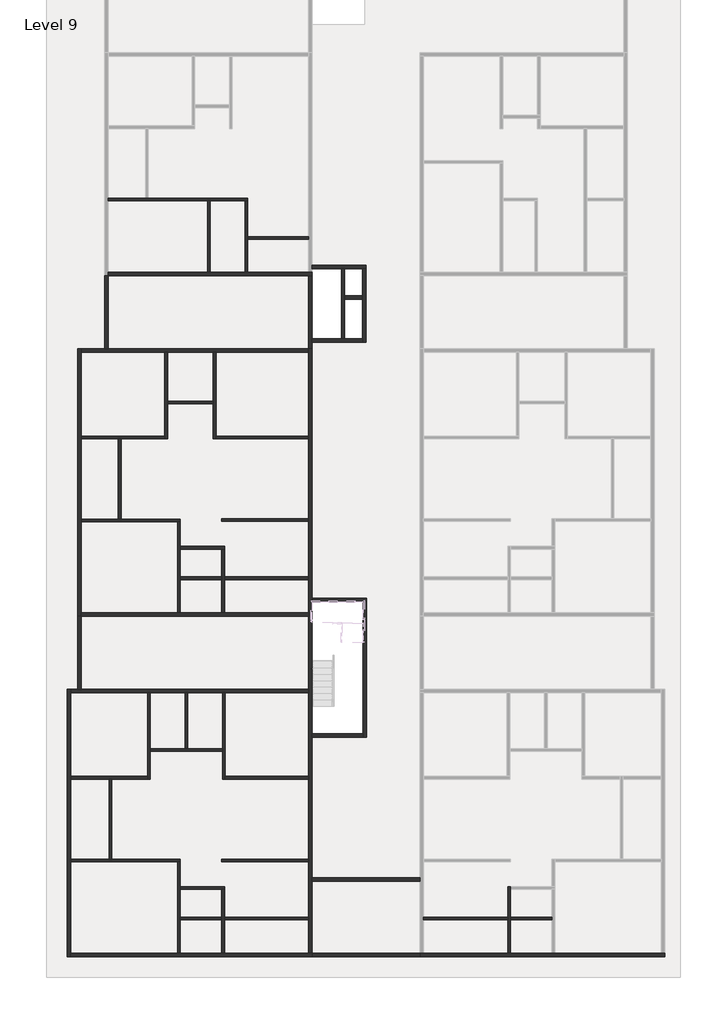
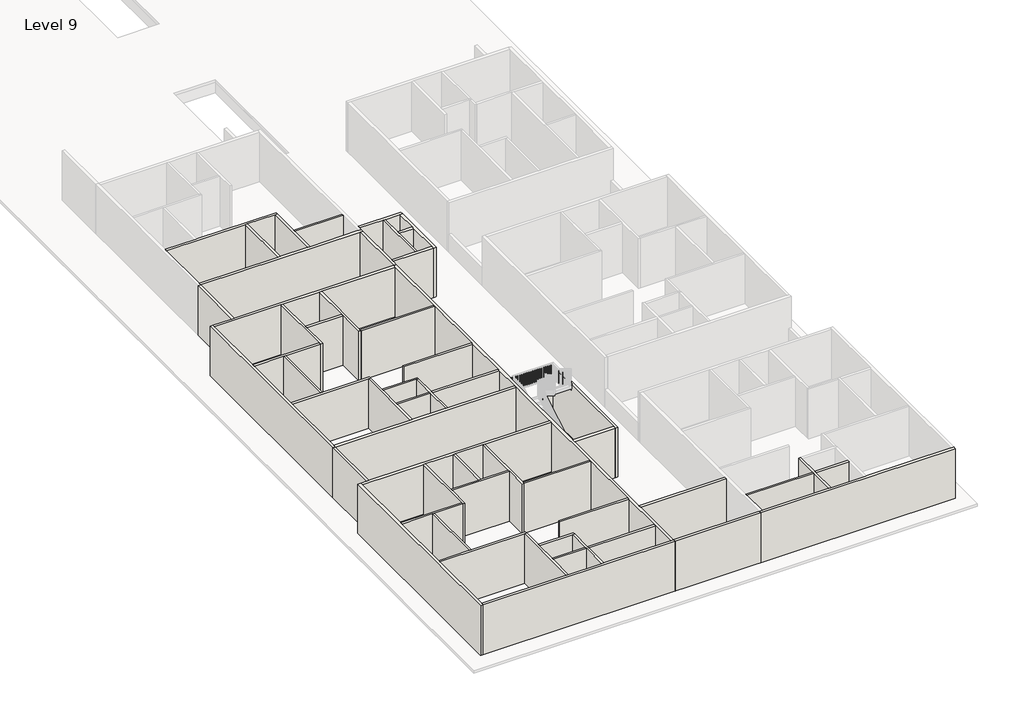
# One storey, part 1 of 8: 55 walls.
"""IFC4 building model written with IfcOpenShell, lengths in millimetres."""

from ifc_helpers import new_model, si_unit, frame, origin, place, context, project, spatial, polyline, outline, extrude, faceted_brep, element, save

model = new_model("IFC4")

# Units and contexts
model_context = context("Model", 3, world=origin())
ifc_project = project(units=[si_unit("LENGTHUNIT", "METRE", prefix="MILLI")], contexts=[model_context])

# Site, building, storey
site = spatial("IfcSite", under=ifc_project)
building = spatial("IfcBuilding", under=site)
storey = spatial("IfcBuildingStorey", under=building, Name="Level 9", Elevation=49618.6172466)

# Walls
placement = place(None, origin())
element("IfcWall", 1, ObjectType="4.5\"", at=placement, inside=storey, context=model_context, shape_type="Brep", body=[
    faceted_brep([(-12531.5544854, -1061.7344126, 49618.6172466), (-8188.1544854, -1061.7344126, 49618.6172466), (-8073.8544854, -1061.7344126, 49618.6172466), (-6549.8544854, -1061.7344126, 49618.6172466), (-6435.5544854, -1061.7344126, 49618.6172466), (-6435.5544854, -1061.7344126, 52666.6172466), (-6549.8544854, -1061.7344126, 52666.6172466), (-8073.8544854, -1061.7344126, 52666.6172466), (-8188.1544854, -1061.7344126, 52666.6172466), (-12531.5544854, -1061.7344126, 52666.6172466), (-12531.5544854, -947.4344126, 49618.6172466), (-12531.5544854, -947.4344126, 52666.6172466), (-10907.2415084, -947.4344126, 52666.6172466), (-10792.9415084, -947.4344126, 52666.6172466), (-6435.5544854, -947.4344126, 52666.6172466), (-6435.5544854, -947.4344126, 49618.6172466), (-10792.9415084, -947.4344126, 49618.6172466), (-10907.2415084, -947.4344126, 49618.6172466)], [[[0, 1, 2, 3, 4, 5, 6, 7, 8, 9]], [[10, 11, 12, 13, 14, 15, 16, 17]], [[4, 3, 2, 1, 0, 10, 17, 16, 15]], [[0, 9, 11, 10]], [[5, 4, 15, 14]], [[9, 8, 7, 6, 5, 14, 13, 12, 11]]]),
])
element("IfcWall", 2, ObjectType="4.5\"", at=placement, inside=storey, context=model_context, shape_type="Brep", body=[
    faceted_brep([(-6549.8544854, -1061.7344126, 49618.6172466), (-6549.8544854, -4185.9344126, 49618.6172466), (-6549.8544854, -4185.9344126, 52666.6172466), (-6549.8544854, -1061.7344126, 52666.6172466), (-6435.5544854, -1061.7344126, 49618.6172466), (-6435.5544854, -1061.7344126, 52666.6172466), (-6435.5544854, -2623.8344126, 52666.6172466), (-6435.5544854, -2738.1344126, 52666.6172466), (-6435.5544854, -4185.9344126, 52666.6172466), (-6435.5544854, -4185.9344126, 49618.6172466), (-6435.5544854, -2738.1344126, 49618.6172466), (-6435.5544854, -2623.8344126, 49618.6172466)], [[[0, 1, 2, 3]], [[4, 5, 6, 7, 8, 9, 10, 11]], [[1, 0, 4, 11, 10, 9]], [[0, 3, 5, 4]], [[2, 1, 9, 8]], [[3, 2, 8, 7, 6, 5]]]),
])
element("IfcWall", 3, ObjectType="4.5\"", at=placement, inside=storey, context=model_context, shape_type="SweptSolid", body=[
    extrude(outline(polyline([(-8188.1544854, -4185.9344126), (-8188.1544854, -1061.7344126), (-8073.8544854, -1061.7344126), (-8073.8544854, -4185.9344126), (-8188.1544854, -4185.9344126)])), frame((0.0, 0.0, 49618.6172466), z_axis=(0.0, 0.0, 1.0), x_axis=(1.0, 0.0, 0.0)), (0.0, 0.0, 1.0), 3048.0),
])
element("IfcWall", 4, ObjectType="4.5\"", at=placement, inside=storey, context=model_context, shape_type="SweptSolid", body=[
    extrude(outline(polyline([(-6435.5544854, -2623.8344126), (-3769.8415084, -2623.8344126), (-3769.8415084, -2738.1344126), (-6435.5544854, -2738.1344126), (-6435.5544854, -2623.8344126)])), frame((0.0, 0.0, 49618.6172466), z_axis=(0.0, 0.0, 1.0), x_axis=(1.0, 0.0, 0.0)), (0.0, 0.0, 1.0), 3048.0),
])
element("IfcWall", 5, ObjectType="4.5\"", at=placement, inside=storey, context=model_context, shape_type="Brep", body=[
    faceted_brep([(-10061.4044854, -7691.1344126, 49618.6172466), (-10061.4044854, -11348.7344126, 49618.6172466), (-10061.4044854, -11463.0344126, 49618.6172466), (-10061.4044854, -11463.0344126, 52666.6172466), (-10061.4044854, -11348.7344126, 52666.6172466), (-10061.4044854, -7691.1344126, 52666.6172466), (-9947.1044854, -7691.1344126, 49618.6172466), (-9947.1044854, -7691.1344126, 52666.6172466), (-9947.1044854, -9824.7344126, 52666.6172466), (-9947.1044854, -9939.0344126, 52666.6172466), (-9947.1044854, -11463.0344126, 52666.6172466), (-9947.1044854, -11463.0344126, 49618.6172466), (-9947.1044854, -9939.0344126, 49618.6172466), (-9947.1044854, -9824.7344126, 49618.6172466)], [[[0, 1, 2, 3, 4, 5]], [[6, 7, 8, 9, 10, 11, 12, 13]], [[2, 1, 0, 6, 13, 12, 11]], [[0, 5, 7, 6]], [[3, 2, 11, 10]], [[5, 4, 3, 10, 9, 8, 7]]]),
])
element("IfcWall", 6, ObjectType="4.5\"", at=placement, inside=storey, context=model_context, shape_type="Brep", body=[
    faceted_brep([(-10061.4044854, -11348.7344126, 49618.6172466), (-13719.0044854, -11348.7344126, 49618.6172466), (-13719.0044854, -11348.7344126, 52666.6172466), (-10061.4044854, -11348.7344126, 52666.6172466), (-10061.4044854, -11463.0344126, 49618.6172466), (-10061.4044854, -11463.0344126, 52666.6172466), (-11980.3915084, -11463.0344126, 52666.6172466), (-12094.6915084, -11463.0344126, 52666.6172466), (-13719.0044854, -11463.0344126, 52666.6172466), (-13719.0044854, -11463.0344126, 49618.6172466), (-12094.6915084, -11463.0344126, 49618.6172466), (-11980.3915084, -11463.0344126, 49618.6172466)], [[[0, 1, 2, 3]], [[4, 5, 6, 7, 8, 9, 10, 11]], [[1, 0, 4, 11, 10, 9]], [[0, 3, 5, 4]], [[2, 1, 9, 8]], [[3, 2, 8, 7, 6, 5]]]),
])
element("IfcWall", 7, ObjectType="4.5\"", at=placement, inside=storey, context=model_context, shape_type="SweptSolid", body=[
    extrude(outline(polyline([(-12094.6915084, -14968.2344126), (-12094.6915084, -11463.0344126), (-11980.3915084, -11463.0344126), (-11980.3915084, -14968.2344126), (-12094.6915084, -14968.2344126)])), frame((0.0, 0.0, 49618.6172466), z_axis=(0.0, 0.0, 1.0), x_axis=(1.0, 0.0, 0.0)), (0.0, 0.0, 1.0), 3048.0),
])
element("IfcWall", 8, ObjectType="4.5\"", at=placement, inside=storey, context=model_context, shape_type="Brep", body=[
    faceted_brep([(-13719.0044854, -15095.2344126, 49618.6172466), (-9510.2415084, -15095.2344126, 49618.6172466), (-9395.9415084, -15095.2344126, 49618.6172466), (-9395.9415084, -15095.2344126, 52666.6172466), (-9510.2415084, -15095.2344126, 52666.6172466), (-13719.0044854, -15095.2344126, 52666.6172466), (-13719.0044854, -14980.9344126, 49618.6172466), (-13719.0044854, -14980.9344126, 52666.6172466), (-9395.9415084, -14980.9344126, 52666.6172466), (-9395.9415084, -14980.9344126, 49618.6172466)], [[[0, 1, 2, 3, 4, 5]], [[6, 7, 8, 9]], [[2, 1, 0, 6, 9]], [[0, 5, 7, 6]], [[3, 2, 9, 8]], [[5, 4, 3, 8, 7]]]),
])
element("IfcWall", 9, ObjectType="4.5\"", at=placement, inside=storey, context=model_context, shape_type="Brep", body=[
    faceted_brep([(-9510.2415084, -15095.2344126, 49618.6172466), (-9510.2415084, -19070.3344126, 49618.6172466), (-9510.2415084, -19070.3344126, 52666.6172466), (-9510.2415084, -15095.2344126, 52666.6172466), (-9395.9415084, -15095.2344126, 49618.6172466), (-9395.9415084, -15095.2344126, 52666.6172466), (-9395.9415084, -16174.7344126, 52666.6172466), (-9395.9415084, -16289.0344126, 52666.6172466), (-9395.9415084, -17508.2344126, 52666.6172466), (-9395.9415084, -17622.5344126, 52666.6172466), (-9395.9415084, -19070.3344126, 52666.6172466), (-9395.9415084, -19070.3344126, 49618.6172466), (-9395.9415084, -17622.5344126, 49618.6172466), (-9395.9415084, -17508.2344126, 49618.6172466), (-9395.9415084, -16289.0344126, 49618.6172466), (-9395.9415084, -16174.7344126, 49618.6172466)], [[[0, 1, 2, 3]], [[4, 5, 6, 7, 8, 9, 10, 11, 12, 13, 14, 15]], [[1, 0, 4, 15, 14, 13, 12, 11]], [[0, 3, 5, 4]], [[2, 1, 11, 10]], [[3, 2, 10, 9, 8, 7, 6, 5]]]),
])
element("IfcWall", 10, ObjectType="4.5\"", at=placement, inside=storey, context=model_context, shape_type="Brep", body=[
    faceted_brep([(-9395.9415084, -16289.0344126, 49618.6172466), (-7567.1415084, -16289.0344126, 49618.6172466), (-7452.8415084, -16289.0344126, 49618.6172466), (-7452.8415084, -16289.0344126, 52666.6172466), (-7567.1415084, -16289.0344126, 52666.6172466), (-9395.9415084, -16289.0344126, 52666.6172466), (-9395.9415084, -16174.7344126, 49618.6172466), (-9395.9415084, -16174.7344126, 52666.6172466), (-7452.8415084, -16174.7344126, 52666.6172466), (-7452.8415084, -16174.7344126, 49618.6172466)], [[[0, 1, 2, 3, 4, 5]], [[6, 7, 8, 9]], [[2, 1, 0, 6, 9]], [[0, 5, 7, 6]], [[3, 2, 9, 8]], [[5, 4, 3, 8, 7]]]),
])
element("IfcWall", 11, ObjectType="4.5\"", at=placement, inside=storey, context=model_context, shape_type="Brep", body=[
    faceted_brep([(-7567.1415084, -16289.0344126, 49618.6172466), (-7567.1415084, -17508.2344126, 49618.6172466), (-7567.1415084, -17622.5344126, 49618.6172466), (-7567.1415084, -19070.3344126, 49618.6172466), (-7567.1415084, -19070.3344126, 52666.6172466), (-7567.1415084, -17622.5344126, 52666.6172466), (-7567.1415084, -17508.2344126, 52666.6172466), (-7567.1415084, -16289.0344126, 52666.6172466), (-7452.8415084, -16289.0344126, 49618.6172466), (-7452.8415084, -16289.0344126, 52666.6172466), (-7452.8415084, -17508.2344126, 52666.6172466), (-7452.8415084, -17622.5344126, 52666.6172466), (-7452.8415084, -19070.3344126, 52666.6172466), (-7452.8415084, -19070.3344126, 49618.6172466), (-7452.8415084, -17622.5344126, 49618.6172466), (-7452.8415084, -17508.2344126, 49618.6172466)], [[[0, 1, 2, 3, 4, 5, 6, 7]], [[8, 9, 10, 11, 12, 13, 14, 15]], [[3, 2, 1, 0, 8, 15, 14, 13]], [[0, 7, 9, 8]], [[4, 3, 13, 12]], [[7, 6, 5, 4, 12, 11, 10, 9]]]),
])
element("IfcWall", 12, ObjectType="4.5\"", at=placement, inside=storey, context=model_context, shape_type="SweptSolid", body=[
    extrude(outline(polyline([(-7567.1415084, -17622.5344126), (-9395.9415084, -17622.5344126), (-9395.9415084, -17508.2344126), (-7567.1415084, -17508.2344126), (-7567.1415084, -17622.5344126)])), frame((0.0, 0.0, 49618.6172466), z_axis=(0.0, 0.0, 1.0), x_axis=(1.0, 0.0, 0.0)), (0.0, 0.0, 1.0), 3048.0),
])
element("IfcWall", 13, ObjectType="4.5\"", at=placement, inside=storey, context=model_context, shape_type="SweptSolid", body=[
    extrude(outline(polyline([(-3769.8415084, -17622.5344126), (-7452.8415084, -17622.5344126), (-7452.8415084, -17508.2344126), (-3769.8415084, -17508.2344126), (-3769.8415084, -17622.5344126)])), frame((0.0, 0.0, 49618.6172466), z_axis=(0.0, 0.0, 1.0), x_axis=(1.0, 0.0, 0.0)), (0.0, 0.0, 1.0), 3048.0),
])
element("IfcWall", 14, ObjectType="4.5\"", at=placement, inside=storey, context=model_context, shape_type="SweptSolid", body=[
    extrude(outline(polyline([(-7567.1415084, -14968.2344126), (-3769.8415084, -14968.2344126), (-3769.8415084, -15082.5344126), (-7567.1415084, -15082.5344126), (-7567.1415084, -14968.2344126)])), frame((0.0, 0.0, 49618.6172466), z_axis=(0.0, 0.0, 1.0), x_axis=(1.0, 0.0, 0.0)), (0.0, 0.0, 1.0), 3048.0),
])
element("IfcWall", 15, ObjectType="4.5\"", at=placement, inside=storey, context=model_context, shape_type="SweptSolid", body=[
    extrude(outline(polyline([(-7940.5044854, -9939.0344126), (-9947.1044854, -9939.0344126), (-9947.1044854, -9824.7344126), (-7940.5044854, -9824.7344126), (-7940.5044854, -9939.0344126)])), frame((0.0, 0.0, 49618.6172466), z_axis=(0.0, 0.0, 1.0), x_axis=(1.0, 0.0, 0.0)), (0.0, 0.0, 1.0), 3048.0),
])
element("IfcWall", 16, ObjectType="4.5\"", at=placement, inside=storey, context=model_context, shape_type="Brep", body=[
    faceted_brep([(-7940.5044854, -7691.1344126, 49618.6172466), (-7940.5044854, -9824.7344126, 49618.6172466), (-7940.5044854, -9939.0344126, 49618.6172466), (-7940.5044854, -11463.0344126, 49618.6172466), (-7940.5044854, -11463.0344126, 52666.6172466), (-7940.5044854, -9939.0344126, 52666.6172466), (-7940.5044854, -9824.7344126, 52666.6172466), (-7940.5044854, -7691.1344126, 52666.6172466), (-7826.2044854, -7691.1344126, 49618.6172466), (-7826.2044854, -7691.1344126, 52666.6172466), (-7826.2044854, -11348.7344126, 52666.6172466), (-7826.2044854, -11463.0344126, 52666.6172466), (-7826.2044854, -11463.0344126, 49618.6172466), (-7826.2044854, -11348.7344126, 49618.6172466)], [[[0, 1, 2, 3, 4, 5, 6, 7]], [[8, 9, 10, 11, 12, 13]], [[3, 2, 1, 0, 8, 13, 12]], [[0, 7, 9, 8]], [[4, 3, 12, 11]], [[7, 6, 5, 4, 11, 10, 9]]]),
])
element("IfcWall", 17, ObjectType="4.5\"", at=placement, inside=storey, context=model_context, shape_type="SweptSolid", body=[
    extrude(outline(polyline([(-3769.8415084, -11463.0344126), (-7826.2044854, -11463.0344126), (-7826.2044854, -11348.7344126), (-3769.8415084, -11348.7344126), (-3769.8415084, -11463.0344126)])), frame((0.0, 0.0, 49618.6172466), z_axis=(0.0, 0.0, 1.0), x_axis=(1.0, 0.0, 0.0)), (0.0, 0.0, 1.0), 3048.0),
])
element("IfcWall", 18, ObjectType="4.5\"", at=placement, inside=storey, context=model_context, shape_type="Brep", body=[
    faceted_brep([(-10818.3415084, -22575.5344126, 49618.6172466), (-10818.3415084, -26233.1344126, 49618.6172466), (-10818.3415084, -26347.4344126, 49618.6172466), (-10818.3415084, -26347.4344126, 52666.6172466), (-10818.3415084, -26233.1344126, 52666.6172466), (-10818.3415084, -22575.5344126, 52666.6172466), (-10704.0415084, -22575.5344126, 49618.6172466), (-10704.0415084, -22575.5344126, 52666.6172466), (-10704.0415084, -25013.9344126, 52666.6172466), (-10704.0415084, -25128.2344126, 52666.6172466), (-10704.0415084, -26347.4344126, 52666.6172466), (-10704.0415084, -26347.4344126, 49618.6172466), (-10704.0415084, -25128.2344126, 49618.6172466), (-10704.0415084, -25013.9344126, 49618.6172466)], [[[0, 1, 2, 3, 4, 5]], [[6, 7, 8, 9, 10, 11, 12, 13]], [[2, 1, 0, 6, 13, 12, 11]], [[0, 5, 7, 6]], [[3, 2, 11, 10]], [[5, 4, 3, 10, 9, 8, 7]]]),
])
element("IfcWall", 19, ObjectType="4.5\"", at=placement, inside=storey, context=model_context, shape_type="Brep", body=[
    faceted_brep([(-10818.3415084, -26233.1344126, 49618.6172466), (-14171.1415084, -26233.1344126, 49618.6172466), (-14171.1415084, -26233.1344126, 52666.6172466), (-10818.3415084, -26233.1344126, 52666.6172466), (-10818.3415084, -26347.4344126, 49618.6172466), (-10818.3415084, -26347.4344126, 52666.6172466), (-12380.4415084, -26347.4344126, 52666.6172466), (-12494.7415084, -26347.4344126, 52666.6172466), (-14171.1415084, -26347.4344126, 52666.6172466), (-14171.1415084, -26347.4344126, 49618.6172466), (-12494.7415084, -26347.4344126, 49618.6172466), (-12380.4415084, -26347.4344126, 49618.6172466)], [[[0, 1, 2, 3]], [[4, 5, 6, 7, 8, 9, 10, 11]], [[1, 0, 4, 11, 10, 9]], [[0, 3, 5, 4]], [[2, 1, 9, 8]], [[3, 2, 8, 7, 6, 5]]]),
])
element("IfcWall", 20, ObjectType="4.5\"", at=placement, inside=storey, context=model_context, shape_type="SweptSolid", body=[
    extrude(outline(polyline([(-9180.0415084, -25013.9344126), (-9180.0415084, -22575.5344126), (-9065.7415084, -22575.5344126), (-9065.7415084, -25013.9344126), (-9180.0415084, -25013.9344126)])), frame((0.0, 0.0, 49618.6172466), z_axis=(0.0, 0.0, 1.0), x_axis=(1.0, 0.0, 0.0)), (0.0, 0.0, 1.0), 3048.0),
])
element("IfcWall", 21, ObjectType="4.5\"", at=placement, inside=storey, context=model_context, shape_type="Brep", body=[
    faceted_brep([(-10704.0415084, -25128.2344126, 49618.6172466), (-7541.7415084, -25128.2344126, 49618.6172466), (-7541.7415084, -25128.2344126, 52666.6172466), (-10704.0415084, -25128.2344126, 52666.6172466), (-10704.0415084, -25013.9344126, 49618.6172466), (-10704.0415084, -25013.9344126, 52666.6172466), (-9180.0415084, -25013.9344126, 52666.6172466), (-9065.7415084, -25013.9344126, 52666.6172466), (-7541.7415084, -25013.9344126, 52666.6172466), (-7541.7415084, -25013.9344126, 49618.6172466), (-9065.7415084, -25013.9344126, 49618.6172466), (-9180.0415084, -25013.9344126, 49618.6172466)], [[[0, 1, 2, 3]], [[4, 5, 6, 7, 8, 9, 10, 11]], [[1, 0, 4, 11, 10, 9]], [[0, 3, 5, 4]], [[2, 1, 9, 8]], [[3, 2, 8, 7, 6, 5]]]),
])
element("IfcWall", 22, ObjectType="4.5\"", at=placement, inside=storey, context=model_context, shape_type="Brep", body=[
    faceted_brep([(-7541.7415084, -22575.5344126, 49618.6172466), (-7541.7415084, -25013.9344126, 49618.6172466), (-7541.7415084, -25128.2344126, 49618.6172466), (-7541.7415084, -26347.4344126, 49618.6172466), (-7541.7415084, -26347.4344126, 52666.6172466), (-7541.7415084, -25128.2344126, 52666.6172466), (-7541.7415084, -25013.9344126, 52666.6172466), (-7541.7415084, -22575.5344126, 52666.6172466), (-7427.4415084, -22575.5344126, 49618.6172466), (-7427.4415084, -22575.5344126, 52666.6172466), (-7427.4415084, -26233.1344126, 52666.6172466), (-7427.4415084, -26347.4344126, 52666.6172466), (-7427.4415084, -26347.4344126, 49618.6172466), (-7427.4415084, -26233.1344126, 49618.6172466)], [[[0, 1, 2, 3, 4, 5, 6, 7]], [[8, 9, 10, 11, 12, 13]], [[3, 2, 1, 0, 8, 13, 12]], [[0, 7, 9, 8]], [[4, 3, 12, 11]], [[7, 6, 5, 4, 11, 10, 9]]]),
])
element("IfcWall", 23, ObjectType="4.5\"", at=placement, inside=storey, context=model_context, shape_type="SweptSolid", body=[
    extrude(outline(polyline([(-3769.8415084, -26347.4344126), (-7427.4415084, -26347.4344126), (-7427.4415084, -26233.1344126), (-3769.8415084, -26233.1344126), (-3769.8415084, -26347.4344126)])), frame((0.0, 0.0, 49618.6172466), z_axis=(0.0, 0.0, 1.0), x_axis=(1.0, 0.0, 0.0)), (0.0, 0.0, 1.0), 3048.0),
])
element("IfcWall", 24, ObjectType="4.5\"", at=placement, inside=storey, context=model_context, shape_type="SweptSolid", body=[
    extrude(outline(polyline([(-12494.7415084, -29852.6344126), (-12494.7415084, -26347.4344126), (-12380.4415084, -26347.4344126), (-12380.4415084, -29852.6344126), (-12494.7415084, -29852.6344126)])), frame((0.0, 0.0, 49618.6172466), z_axis=(0.0, 0.0, 1.0), x_axis=(1.0, 0.0, 0.0)), (0.0, 0.0, 1.0), 3048.0),
])
element("IfcWall", 25, ObjectType="4.5\"", at=placement, inside=storey, context=model_context, shape_type="Brep", body=[
    faceted_brep([(-14171.1415084, -29966.9344126, 49618.6172466), (-9510.2415084, -29966.9344126, 49618.6172466), (-9395.9415084, -29966.9344126, 49618.6172466), (-9395.9415084, -29966.9344126, 52666.6172466), (-9510.2415084, -29966.9344126, 52666.6172466), (-14171.1415084, -29966.9344126, 52666.6172466), (-14171.1415084, -29852.6344126, 49618.6172466), (-14171.1415084, -29852.6344126, 52666.6172466), (-12494.7415084, -29852.6344126, 52666.6172466), (-12380.4415084, -29852.6344126, 52666.6172466), (-9395.9415084, -29852.6344126, 52666.6172466), (-9395.9415084, -29852.6344126, 49618.6172466), (-12380.4415084, -29852.6344126, 49618.6172466), (-12494.7415084, -29852.6344126, 49618.6172466)], [[[0, 1, 2, 3, 4, 5]], [[6, 7, 8, 9, 10, 11, 12, 13]], [[2, 1, 0, 6, 13, 12, 11]], [[0, 5, 7, 6]], [[3, 2, 11, 10]], [[5, 4, 3, 10, 9, 8, 7]]]),
])
element("IfcWall", 26, ObjectType="4.5\"", at=placement, inside=storey, context=model_context, shape_type="Brep", body=[
    faceted_brep([(-9510.2415084, -29966.9344126, 49618.6172466), (-9510.2415084, -33954.7344126, 49618.6172466), (-9510.2415084, -33954.7344126, 52666.6172466), (-9510.2415084, -29966.9344126, 52666.6172466), (-9395.9415084, -29966.9344126, 49618.6172466), (-9395.9415084, -29966.9344126, 52666.6172466), (-9395.9415084, -31059.1344126, 52666.6172466), (-9395.9415084, -31173.4344126, 52666.6172466), (-9395.9415084, -32392.6344126, 52666.6172466), (-9395.9415084, -32506.9344126, 52666.6172466), (-9395.9415084, -33954.7344126, 52666.6172466), (-9395.9415084, -33954.7344126, 49618.6172466), (-9395.9415084, -32506.9344126, 49618.6172466), (-9395.9415084, -32392.6344126, 49618.6172466), (-9395.9415084, -31173.4344126, 49618.6172466), (-9395.9415084, -31059.1344126, 49618.6172466)], [[[0, 1, 2, 3]], [[4, 5, 6, 7, 8, 9, 10, 11, 12, 13, 14, 15]], [[1, 0, 4, 15, 14, 13, 12, 11]], [[0, 3, 5, 4]], [[2, 1, 11, 10]], [[3, 2, 10, 9, 8, 7, 6, 5]]]),
])
element("IfcWall", 27, ObjectType="4.5\"", at=placement, inside=storey, context=model_context, shape_type="Brep", body=[
    faceted_brep([(-9395.9415084, -31173.4344126, 49618.6172466), (-7567.1415084, -31173.4344126, 49618.6172466), (-7452.8415084, -31173.4344126, 49618.6172466), (-7452.8415084, -31173.4344126, 52666.6172466), (-7567.1415084, -31173.4344126, 52666.6172466), (-9395.9415084, -31173.4344126, 52666.6172466), (-9395.9415084, -31059.1344126, 49618.6172466), (-9395.9415084, -31059.1344126, 52666.6172466), (-7452.8415084, -31059.1344126, 52666.6172466), (-7452.8415084, -31059.1344126, 49618.6172466)], [[[0, 1, 2, 3, 4, 5]], [[6, 7, 8, 9]], [[2, 1, 0, 6, 9]], [[0, 5, 7, 6]], [[3, 2, 9, 8]], [[5, 4, 3, 8, 7]]]),
])
element("IfcWall", 28, ObjectType="4.5\"", at=placement, inside=storey, context=model_context, shape_type="Brep", body=[
    faceted_brep([(-7567.1415084, -31173.4344126, 49618.6172466), (-7567.1415084, -32392.6344126, 49618.6172466), (-7567.1415084, -32506.9344126, 49618.6172466), (-7567.1415084, -33954.7344126, 49618.6172466), (-7567.1415084, -33954.7344126, 52666.6172466), (-7567.1415084, -32506.9344126, 52666.6172466), (-7567.1415084, -32392.6344126, 52666.6172466), (-7567.1415084, -31173.4344126, 52666.6172466), (-7452.8415084, -31173.4344126, 49618.6172466), (-7452.8415084, -31173.4344126, 52666.6172466), (-7452.8415084, -32392.6344126, 52666.6172466), (-7452.8415084, -32506.9344126, 52666.6172466), (-7452.8415084, -33954.7344126, 52666.6172466), (-7452.8415084, -33954.7344126, 49618.6172466), (-7452.8415084, -32506.9344126, 49618.6172466), (-7452.8415084, -32392.6344126, 49618.6172466)], [[[0, 1, 2, 3, 4, 5, 6, 7]], [[8, 9, 10, 11, 12, 13, 14, 15]], [[3, 2, 1, 0, 8, 15, 14, 13]], [[0, 7, 9, 8]], [[4, 3, 13, 12]], [[7, 6, 5, 4, 12, 11, 10, 9]]]),
])
element("IfcWall", 29, ObjectType="4.5\"", at=placement, inside=storey, context=model_context, shape_type="SweptSolid", body=[
    extrude(outline(polyline([(-3769.8415084, -32392.6344126), (-3769.8415084, -32506.9344126), (-7452.8415084, -32506.9344126), (-7452.8415084, -32392.6344126), (-3769.8415084, -32392.6344126)])), frame((0.0, 0.0, 49618.6172466), z_axis=(0.0, 0.0, 1.0), x_axis=(1.0, 0.0, 0.0)), (0.0, 0.0, 1.0), 3048.0),
    extrude(outline(polyline([(-9395.9415084, -32506.9344126), (-9395.9415084, -32392.6344126), (-7567.1415084, -32392.6344126), (-7567.1415084, -32506.9344126), (-9395.9415084, -32506.9344126)])), frame((0.0, 0.0, 49618.6172466), z_axis=(0.0, 0.0, 1.0), x_axis=(1.0, 0.0, 0.0)), (0.0, 0.0, 1.0), 3048.0),
])
element("IfcWall", 30, ObjectType="4.5\"", at=placement, inside=storey, context=model_context, shape_type="SweptSolid", body=[
    extrude(outline(polyline([(-7567.1415084, -29852.6344126), (-3769.8415084, -29852.6344126), (-3769.8415084, -29966.9344126), (-7567.1415084, -29966.9344126), (-7567.1415084, -29852.6344126)])), frame((0.0, 0.0, 49618.6172466), z_axis=(0.0, 0.0, 1.0), x_axis=(1.0, 0.0, 0.0)), (0.0, 0.0, 1.0), 3048.0),
])
element("IfcWall", 31, ObjectType="4.5\"", at=placement, inside=storey, context=model_context, shape_type="SweptSolid", body=[
    extrude(outline(polyline([(4942.3584916, -32506.9344126), (1259.3584916, -32506.9344126), (1259.3584916, -32392.6344126), (4942.3584916, -32392.6344126), (4942.3584916, -32506.9344126)])), frame((0.0, 0.0, 49618.6172466), z_axis=(0.0, 0.0, 1.0), x_axis=(1.0, 0.0, 0.0)), (0.0, 0.0, 1.0), 3048.0),
])
element("IfcWall", 32, ObjectType="4.5\"", at=placement, inside=storey, context=model_context, shape_type="Brep", body=[
    faceted_brep([(4942.3584916, -31059.1344126, 49618.6172466), (4942.3584916, -32392.6344126, 49618.6172466), (4942.3584916, -32506.9344126, 49618.6172466), (4942.3584916, -33954.7344126, 49618.6172466), (4942.3584916, -33954.7344126, 52666.6172466), (4942.3584916, -32506.9344126, 52666.6172466), (4942.3584916, -32392.6344126, 52666.6172466), (4942.3584916, -31059.1344126, 52666.6172466), (5056.6584916, -31059.1344126, 49618.6172466), (5056.6584916, -31059.1344126, 52666.6172466), (5056.6584916, -31173.4344126, 52666.6172466), (5056.6584916, -32392.6344126, 52666.6172466), (5056.6584916, -32506.9344126, 52666.6172466), (5056.6584916, -33954.7344126, 52666.6172466), (5056.6584916, -33954.7344126, 49618.6172466), (5056.6584916, -32506.9344126, 49618.6172466), (5056.6584916, -32392.6344126, 49618.6172466), (5056.6584916, -31173.4344126, 49618.6172466)], [[[0, 1, 2, 3, 4, 5, 6, 7]], [[8, 9, 10, 11, 12, 13, 14, 15, 16, 17]], [[3, 2, 1, 0, 8, 17, 16, 15, 14]], [[4, 3, 14, 13]], [[0, 7, 9, 8]], [[7, 6, 5, 4, 13, 12, 11, 10, 9]]]),
])
element("IfcWall", 33, ObjectType="4.5\"", at=placement, inside=storey, context=model_context, shape_type="SweptSolid", body=[
    extrude(outline(polyline([(6885.4584916, -32506.9344126), (5056.6584916, -32506.9344126), (5056.6584916, -32392.6344126), (6885.4584916, -32392.6344126), (6885.4584916, -32506.9344126)])), frame((0.0, 0.0, 49618.6172466), z_axis=(0.0, 0.0, 1.0), x_axis=(1.0, 0.0, 0.0)), (0.0, 0.0, 1.0), 3048.0),
])
element("IfcWall", 34, ObjectType="4.5\"", at=placement, inside=storey, context=model_context, shape_type="Brep", body=[
    faceted_brep([(-2207.6738684, -7082.6751812, 49618.6172466), (-2207.6738684, -5366.3479894, 49618.6172466), (-2207.6738684, -5213.9479894, 49618.6172466), (-2207.6738684, -4034.6751812, 49618.6172466), (-2207.6738684, -4034.6751812, 52666.6172466), (-2207.6738684, -5213.9479894, 52666.6172466), (-2207.6738684, -5366.3479894, 52666.6172466), (-2207.6738684, -7082.6751812, 52666.6172466), (-2321.9738684, -7082.6751812, 49618.6172466), (-2321.9738684, -7082.6751812, 52666.6172466), (-2321.9738684, -4034.6751812, 52666.6172466), (-2321.9738684, -4034.6751812, 49618.6172466)], [[[0, 1, 2, 3, 4, 5, 6, 7]], [[8, 9, 10, 11]], [[3, 2, 1, 0, 8, 11]], [[7, 6, 5, 4, 10, 9]], [[4, 3, 11, 10]], [[0, 7, 9, 8]]]),
])
element("IfcWall", 35, ObjectType="6\"", at=placement, inside=storey, context=model_context, shape_type="Brep", body=[
    faceted_brep([(-12531.5544854, -4338.3344126, 49618.6172466), (-3769.8415084, -4338.3344126, 49618.6172466), (-3617.4415084, -4338.3344126, 49618.6172466), (-3617.4415084, -4338.3344126, 52666.6172466), (-3769.8415084, -4338.3344126, 52666.6172466), (-12531.5544854, -4338.3344126, 52666.6172466), (-12531.5544854, -4185.9344126, 49618.6172466), (-12531.5544854, -4185.9344126, 52666.6172466), (-8188.1544854, -4185.9344126, 52666.6172466), (-8073.8544854, -4185.9344126, 52666.6172466), (-6549.8544854, -4185.9344126, 52666.6172466), (-6435.5544854, -4185.9344126, 52666.6172466), (-3769.8415084, -4185.9344126, 52666.6172466), (-3617.4415084, -4185.9344126, 52666.6172466), (-3617.4415084, -4185.9344126, 49618.6172466), (-3769.8415084, -4185.9344126, 49618.6172466), (-6435.5544854, -4185.9344126, 49618.6172466), (-6549.8544854, -4185.9344126, 49618.6172466), (-8073.8544854, -4185.9344126, 49618.6172466), (-8188.1544854, -4185.9344126, 49618.6172466)], [[[0, 1, 2, 3, 4, 5]], [[6, 7, 8, 9, 10, 11, 12, 13, 14, 15, 16, 17, 18, 19]], [[2, 1, 0, 6, 19, 18, 17, 16, 15, 14]], [[0, 5, 7, 6]], [[3, 2, 14, 13]], [[5, 4, 3, 13, 12, 11, 10, 9, 8, 7]]]),
])
element("IfcWall", 36, ObjectType="6\"", at=placement, inside=storey, context=model_context, shape_type="Brep", body=[
    faceted_brep([(-13871.4044854, -7538.7344126, 49618.6172466), (-13871.4044854, -19222.7344126, 49618.6172466), (-13871.4044854, -19222.7344126, 52666.6172466), (-13871.4044854, -7538.7344126, 52666.6172466), (-13719.0044854, -7538.7344126, 49618.6172466), (-13719.0044854, -7538.7344126, 52666.6172466), (-13719.0044854, -7691.1344126, 52666.6172466), (-13719.0044854, -11348.7344126, 52666.6172466), (-13719.0044854, -11463.0344126, 52666.6172466), (-13719.0044854, -14980.9344126, 52666.6172466), (-13719.0044854, -15095.2344126, 52666.6172466), (-13719.0044854, -19070.3344126, 52666.6172466), (-13719.0044854, -19222.7344126, 52666.6172466), (-13719.0044854, -19222.7344126, 49618.6172466), (-13719.0044854, -19070.3344126, 49618.6172466), (-13719.0044854, -15095.2344126, 49618.6172466), (-13719.0044854, -14980.9344126, 49618.6172466), (-13719.0044854, -11463.0344126, 49618.6172466), (-13719.0044854, -11348.7344126, 49618.6172466), (-13719.0044854, -7691.1344126, 49618.6172466)], [[[0, 1, 2, 3]], [[4, 5, 6, 7, 8, 9, 10, 11, 12, 13, 14, 15, 16, 17, 18, 19]], [[1, 0, 4, 19, 18, 17, 16, 15, 14, 13]], [[2, 1, 13, 12]], [[0, 3, 5, 4]], [[3, 2, 12, 11, 10, 9, 8, 7, 6, 5]]]),
])
element("IfcWall", 37, ObjectType="6\"", at=placement, inside=storey, context=model_context, shape_type="Brep", body=[
    faceted_brep([(-13719.0044854, -19222.7344126, 49618.6172466), (-3769.8415084, -19222.7344126, 49618.6172466), (-3769.8415084, -19222.7344126, 52666.6172466), (-13719.0044854, -19222.7344126, 52666.6172466), (-13719.0044854, -19070.3344126, 49618.6172466), (-13719.0044854, -19070.3344126, 52666.6172466), (-9510.2415084, -19070.3344126, 52666.6172466), (-9395.9415084, -19070.3344126, 52666.6172466), (-7567.1415084, -19070.3344126, 52666.6172466), (-7452.8415084, -19070.3344126, 52666.6172466), (-3769.8415084, -19070.3344126, 52666.6172466), (-3769.8415084, -19070.3344126, 49618.6172466), (-7452.8415084, -19070.3344126, 49618.6172466), (-7567.1415084, -19070.3344126, 49618.6172466), (-9395.9415084, -19070.3344126, 49618.6172466), (-9510.2415084, -19070.3344126, 49618.6172466)], [[[0, 1, 2, 3]], [[4, 5, 6, 7, 8, 9, 10, 11, 12, 13, 14, 15]], [[1, 0, 4, 15, 14, 13, 12, 11]], [[0, 3, 5, 4]], [[2, 1, 11, 10]], [[3, 2, 10, 9, 8, 7, 6, 5]]]),
])
element("IfcWall", 38, ObjectType="6\"", at=placement, inside=storey, context=model_context, shape_type="Brep", body=[
    faceted_brep([(-3617.4415084, -33954.7344126, 49618.6172466), (-3617.4415084, -30820.9325185, 49618.6172466), (-3617.4415084, -30668.5325185, 49618.6172466), (-3617.4415084, -24525.9851539, 49618.6172466), (-3617.4415084, -24373.5851539, 49618.6172466), (-3617.4415084, -18582.3851539, 49618.6172466), (-3617.4415084, -18429.9851539, 49618.6172466), (-3617.4415084, -7538.7344126, 49618.6172466), (-3617.4415084, -7538.7344126, 52666.6172466), (-3617.4415084, -18429.9851539, 52666.6172466), (-3617.4415084, -18582.3851539, 52666.6172466), (-3617.4415084, -24373.5851539, 52666.6172466), (-3617.4415084, -24525.9851539, 52666.6172466), (-3617.4415084, -30668.5325185, 52666.6172466), (-3617.4415084, -30820.9325185, 52666.6172466), (-3617.4415084, -33954.7344126, 52666.6172466), (-3769.8415084, -33954.7344126, 49618.6172466), (-3769.8415084, -33954.7344126, 52666.6172466), (-3769.8415084, -32506.9344126, 52666.6172466), (-3769.8415084, -32392.6344126, 52666.6172466), (-3769.8415084, -29966.9344126, 52666.6172466), (-3769.8415084, -29852.6344126, 52666.6172466), (-3769.8415084, -26347.4344126, 52666.6172466), (-3769.8415084, -26233.1344126, 52666.6172466), (-3769.8415084, -22575.5344126, 52666.6172466), (-3769.8415084, -22423.1344126, 52666.6172466), (-3769.8415084, -19222.7344126, 52666.6172466), (-3769.8415084, -19070.3344126, 52666.6172466), (-3769.8415084, -17622.5344126, 52666.6172466), (-3769.8415084, -17508.2344126, 52666.6172466), (-3769.8415084, -15082.5344126, 52666.6172466), (-3769.8415084, -14968.2344126, 52666.6172466), (-3769.8415084, -11463.0344126, 52666.6172466), (-3769.8415084, -11348.7344126, 52666.6172466), (-3769.8415084, -7691.1344126, 52666.6172466), (-3769.8415084, -7538.7344126, 52666.6172466), (-3769.8415084, -7538.7344126, 49618.6172466), (-3769.8415084, -7691.1344126, 49618.6172466), (-3769.8415084, -11348.7344126, 49618.6172466), (-3769.8415084, -11463.0344126, 49618.6172466), (-3769.8415084, -14968.2344126, 49618.6172466), (-3769.8415084, -15082.5344126, 49618.6172466), (-3769.8415084, -17508.2344126, 49618.6172466), (-3769.8415084, -17622.5344126, 49618.6172466), (-3769.8415084, -19070.3344126, 49618.6172466), (-3769.8415084, -19222.7344126, 49618.6172466), (-3769.8415084, -22423.1344126, 49618.6172466), (-3769.8415084, -22575.5344126, 49618.6172466), (-3769.8415084, -26233.1344126, 49618.6172466), (-3769.8415084, -26347.4344126, 49618.6172466), (-3769.8415084, -29852.6344126, 49618.6172466), (-3769.8415084, -29966.9344126, 49618.6172466), (-3769.8415084, -32392.6344126, 49618.6172466), (-3769.8415084, -32506.9344126, 49618.6172466)], [[[0, 1, 2, 3, 4, 5, 6, 7, 8, 9, 10, 11, 12, 13, 14, 15]], [[16, 17, 18, 19, 20, 21, 22, 23, 24, 25, 26, 27, 28, 29, 30, 31, 32, 33, 34, 35, 36, 37, 38, 39, 40, 41, 42, 43, 44, 45, 46, 47, 48, 49, 50, 51, 52, 53]], [[7, 6, 5, 4, 3, 2, 1, 0, 16, 53, 52, 51, 50, 49, 48, 47, 46, 45, 44, 43, 42, 41, 40, 39, 38, 37, 36]], [[8, 7, 36, 35]], [[0, 15, 17, 16]], [[15, 14, 13, 12, 11, 10, 9, 8, 35, 34, 33, 32, 31, 30, 29, 28, 27, 26, 25, 24, 23, 22, 21, 20, 19, 18, 17]]]),
])
element("IfcWall", 39, ObjectType="6\"", at=placement, inside=storey, context=model_context, shape_type="Brep", body=[
    faceted_brep([(-3769.8415084, -7538.7344126, 49618.6172466), (-12531.5544854, -7538.7344126, 49618.6172466), (-12683.9544854, -7538.7344126, 49618.6172466), (-13719.0044854, -7538.7344126, 49618.6172466), (-13719.0044854, -7538.7344126, 52666.6172466), (-12683.9544854, -7538.7344126, 52666.6172466), (-12531.5544854, -7538.7344126, 52666.6172466), (-3769.8415084, -7538.7344126, 52666.6172466), (-3769.8415084, -7691.1344126, 49618.6172466), (-3769.8415084, -7691.1344126, 52666.6172466), (-7826.2044854, -7691.1344126, 52666.6172466), (-7940.5044854, -7691.1344126, 52666.6172466), (-9947.1044854, -7691.1344126, 52666.6172466), (-10061.4044854, -7691.1344126, 52666.6172466), (-13719.0044854, -7691.1344126, 52666.6172466), (-13719.0044854, -7691.1344126, 49618.6172466), (-10061.4044854, -7691.1344126, 49618.6172466), (-9947.1044854, -7691.1344126, 49618.6172466), (-7940.5044854, -7691.1344126, 49618.6172466), (-7826.2044854, -7691.1344126, 49618.6172466)], [[[0, 1, 2, 3, 4, 5, 6, 7]], [[8, 9, 10, 11, 12, 13, 14, 15, 16, 17, 18, 19]], [[3, 2, 1, 0, 8, 19, 18, 17, 16, 15]], [[0, 7, 9, 8]], [[4, 3, 15, 14]], [[7, 6, 5, 4, 14, 13, 12, 11, 10, 9]]]),
])
element("IfcWall", 40, ObjectType="6\"", at=placement, inside=storey, context=model_context, shape_type="Brep", body=[
    faceted_brep([(-14323.5415084, -22423.1344126, 49618.6172466), (-14323.5415084, -34107.1344126, 49618.6172466), (-14323.5415084, -34107.1344126, 52666.6172466), (-14323.5415084, -22423.1344126, 52666.6172466), (-14171.1415084, -22423.1344126, 49618.6172466), (-14171.1415084, -22423.1344126, 52666.6172466), (-14171.1415084, -22575.5344126, 52666.6172466), (-14171.1415084, -26233.1344126, 52666.6172466), (-14171.1415084, -26347.4344126, 52666.6172466), (-14171.1415084, -29852.6344126, 52666.6172466), (-14171.1415084, -29966.9344126, 52666.6172466), (-14171.1415084, -33954.7344126, 52666.6172466), (-14171.1415084, -34107.1344126, 52666.6172466), (-14171.1415084, -34107.1344126, 49618.6172466), (-14171.1415084, -33954.7344126, 49618.6172466), (-14171.1415084, -29966.9344126, 49618.6172466), (-14171.1415084, -29852.6344126, 49618.6172466), (-14171.1415084, -26347.4344126, 49618.6172466), (-14171.1415084, -26233.1344126, 49618.6172466), (-14171.1415084, -22575.5344126, 49618.6172466)], [[[0, 1, 2, 3]], [[4, 5, 6, 7, 8, 9, 10, 11, 12, 13, 14, 15, 16, 17, 18, 19]], [[1, 0, 4, 19, 18, 17, 16, 15, 14, 13]], [[2, 1, 13, 12]], [[0, 3, 5, 4]], [[3, 2, 12, 11, 10, 9, 8, 7, 6, 5]]]),
])
element("IfcWall", 41, ObjectType="6\"", at=placement, inside=storey, context=model_context, shape_type="Brep", body=[
    faceted_brep([(-14171.1415084, -34107.1344126, 49618.6172466), (-3617.4415084, -34107.1344126, 49618.6172466), (-3617.4415084, -34107.1344126, 52666.6172466), (-14171.1415084, -34107.1344126, 52666.6172466), (-14171.1415084, -33954.7344126, 49618.6172466), (-14171.1415084, -33954.7344126, 52666.6172466), (-9510.2415084, -33954.7344126, 52666.6172466), (-9395.9415084, -33954.7344126, 52666.6172466), (-7567.1415084, -33954.7344126, 52666.6172466), (-7452.8415084, -33954.7344126, 52666.6172466), (-3769.8415084, -33954.7344126, 52666.6172466), (-3617.4415084, -33954.7344126, 52666.6172466), (-3617.4415084, -33954.7344126, 49618.6172466), (-3769.8415084, -33954.7344126, 49618.6172466), (-7452.8415084, -33954.7344126, 49618.6172466), (-7567.1415084, -33954.7344126, 49618.6172466), (-9395.9415084, -33954.7344126, 49618.6172466), (-9510.2415084, -33954.7344126, 49618.6172466)], [[[0, 1, 2, 3]], [[4, 5, 6, 7, 8, 9, 10, 11, 12, 13, 14, 15, 16, 17]], [[1, 0, 4, 17, 16, 15, 14, 13, 12]], [[0, 3, 5, 4]], [[2, 1, 12, 11]], [[3, 2, 11, 10, 9, 8, 7, 6, 5]]]),
])
element("IfcWall", 42, ObjectType="6\"", at=placement, inside=storey, context=model_context, shape_type="Brep", body=[
    faceted_brep([(-3769.8415084, -22423.1344126, 49618.6172466), (-13719.0044854, -22423.1344126, 49618.6172466), (-13871.4044854, -22423.1344126, 49618.6172466), (-14171.1415084, -22423.1344126, 49618.6172466), (-14171.1415084, -22423.1344126, 52666.6172466), (-13871.4044854, -22423.1344126, 52666.6172466), (-13719.0044854, -22423.1344126, 52666.6172466), (-3769.8415084, -22423.1344126, 52666.6172466), (-3769.8415084, -22575.5344126, 49618.6172466), (-3769.8415084, -22575.5344126, 52666.6172466), (-7427.4415084, -22575.5344126, 52666.6172466), (-7541.7415084, -22575.5344126, 52666.6172466), (-9065.7415084, -22575.5344126, 52666.6172466), (-9180.0415084, -22575.5344126, 52666.6172466), (-10704.0415084, -22575.5344126, 52666.6172466), (-10818.3415084, -22575.5344126, 52666.6172466), (-14171.1415084, -22575.5344126, 52666.6172466), (-14171.1415084, -22575.5344126, 49618.6172466), (-10818.3415084, -22575.5344126, 49618.6172466), (-10704.0415084, -22575.5344126, 49618.6172466), (-9180.0415084, -22575.5344126, 49618.6172466), (-9065.7415084, -22575.5344126, 49618.6172466), (-7541.7415084, -22575.5344126, 49618.6172466), (-7427.4415084, -22575.5344126, 49618.6172466)], [[[0, 1, 2, 3, 4, 5, 6, 7]], [[8, 9, 10, 11, 12, 13, 14, 15, 16, 17, 18, 19, 20, 21, 22, 23]], [[3, 2, 1, 0, 8, 23, 22, 21, 20, 19, 18, 17]], [[0, 7, 9, 8]], [[4, 3, 17, 16]], [[7, 6, 5, 4, 16, 15, 14, 13, 12, 11, 10, 9]]]),
])
element("IfcWall", 43, ObjectType="6\"", at=placement, inside=storey, context=model_context, shape_type="Brep", body=[
    faceted_brep([(1106.9584916, -34107.1344126, 49618.6172466), (11813.0584916, -34107.1344126, 49618.6172466), (11813.0584916, -34107.1344126, 52666.6172466), (1106.9584916, -34107.1344126, 52666.6172466), (1106.9584916, -33954.7344126, 49618.6172466), (1106.9584916, -33954.7344126, 52666.6172466), (1259.3584916, -33954.7344126, 52666.6172466), (4942.3584916, -33954.7344126, 52666.6172466), (5056.6584916, -33954.7344126, 52666.6172466), (6885.4584916, -33954.7344126, 52666.6172466), (6999.7584916, -33954.7344126, 52666.6172466), (11660.6584916, -33954.7344126, 52666.6172466), (11813.0584916, -33954.7344126, 52666.6172466), (11813.0584916, -33954.7344126, 49618.6172466), (11660.6584916, -33954.7344126, 49618.6172466), (6999.7584916, -33954.7344126, 49618.6172466), (6885.4584916, -33954.7344126, 49618.6172466), (5056.6584916, -33954.7344126, 49618.6172466), (4942.3584916, -33954.7344126, 49618.6172466), (1259.3584916, -33954.7344126, 49618.6172466)], [[[0, 1, 2, 3]], [[4, 5, 6, 7, 8, 9, 10, 11, 12, 13, 14, 15, 16, 17, 18, 19]], [[1, 0, 4, 19, 18, 17, 16, 15, 14, 13]], [[2, 1, 13, 12]], [[0, 3, 5, 4]], [[3, 2, 12, 11, 10, 9, 8, 7, 6, 5]]]),
])
element("IfcWall", 44, ObjectType="6\"", at=placement, inside=storey, context=model_context, shape_type="Brep", body=[
    faceted_brep([(-3617.4415084, -18582.3851539, 49618.6172466), (-1382.2415084, -18582.3851539, 49618.6172466), (-1229.8415084, -18582.3851539, 49618.6172466), (-1229.8415084, -18582.3851539, 52666.6172466), (-1382.2415084, -18582.3851539, 52666.6172466), (-3617.4415084, -18582.3851539, 52666.6172466), (-3617.4415084, -18429.9851539, 49618.6172466), (-3617.4415084, -18429.9851539, 52666.6172466), (-1229.8415084, -18429.9851539, 52666.6172466), (-1229.8415084, -18429.9851539, 49618.6172466)], [[[0, 1, 2, 3, 4, 5]], [[6, 7, 8, 9]], [[2, 1, 0, 6, 9]], [[5, 4, 3, 8, 7]], [[0, 5, 7, 6]], [[3, 2, 9, 8]]]),
])
element("IfcWall", 45, ObjectType="6\"", at=placement, inside=storey, context=model_context, shape_type="Brep", body=[
    faceted_brep([(-1382.2415084, -18582.3851539, 49618.6172466), (-1382.2415084, -24373.5851539, 49618.6172466), (-1382.2415084, -24525.9851539, 49618.6172466), (-1382.2415084, -24525.9851539, 52666.6172466), (-1382.2415084, -24373.5851539, 52666.6172466), (-1382.2415084, -18582.3851539, 52666.6172466), (-1229.8415084, -18582.3851539, 49618.6172466), (-1229.8415084, -18582.3851539, 52666.6172466), (-1229.8415084, -24525.9851539, 52666.6172466), (-1229.8415084, -24525.9851539, 49618.6172466)], [[[0, 1, 2, 3, 4, 5]], [[6, 7, 8, 9]], [[2, 1, 0, 6, 9]], [[5, 4, 3, 8, 7]], [[0, 5, 7, 6]], [[3, 2, 9, 8]]]),
])
element("IfcWall", 46, ObjectType="6\"", at=placement, inside=storey, context=model_context, shape_type="SweptSolid", body=[
    extrude(outline(polyline([(-3617.4415084, -24373.5851539), (-1382.2415084, -24373.5851539), (-1382.2415084, -24525.9851539), (-3617.4415084, -24525.9851539), (-3617.4415084, -24373.5851539)])), frame((0.0, 0.0, 49618.6172466), z_axis=(0.0, 0.0, 1.0), x_axis=(1.0, 0.0, 0.0)), (0.0, 0.0, 1.0), 3048.0),
])
element("IfcWall", 47, ObjectType="6\"", at=placement, inside=storey, context=model_context, shape_type="Brep", body=[
    faceted_brep([(-3769.8415084, -4338.3344126, 49618.6172466), (-3769.8415084, -7538.7344126, 49618.6172466), (-3769.8415084, -7538.7344126, 52666.6172466), (-3769.8415084, -4338.3344126, 52666.6172466), (-3617.4415084, -4338.3344126, 49618.6172466), (-3617.4415084, -4338.3344126, 52666.6172466), (-3617.4415084, -7082.6751812, 52666.6172466), (-3617.4415084, -7235.0751812, 52666.6172466), (-3617.4415084, -7538.7344126, 52666.6172466), (-3617.4415084, -7538.7344126, 49618.6172466), (-3617.4415084, -7235.0751812, 49618.6172466), (-3617.4415084, -7082.6751812, 49618.6172466)], [[[0, 1, 2, 3]], [[4, 5, 6, 7, 8, 9, 10, 11]], [[1, 0, 4, 11, 10, 9]], [[0, 3, 5, 4]], [[2, 1, 9, 8]], [[3, 2, 8, 7, 6, 5]]]),
])
element("IfcWall", 48, ObjectType="6\"", at=placement, inside=storey, context=model_context, shape_type="Brep", body=[
    faceted_brep([(-3617.4415084, -4034.6751812, 49618.6172466), (-2321.9738684, -4034.6751812, 49618.6172466), (-2207.6738684, -4034.6751812, 49618.6172466), (-1407.6415084, -4034.6751812, 49618.6172466), (-1255.2415084, -4034.6751812, 49618.6172466), (-1255.2415084, -4034.6751812, 52666.6172466), (-1407.6415084, -4034.6751812, 52666.6172466), (-2207.6738684, -4034.6751812, 52666.6172466), (-2321.9738684, -4034.6751812, 52666.6172466), (-3617.4415084, -4034.6751812, 52666.6172466), (-3617.4415084, -3882.2751812, 49618.6172466), (-3617.4415084, -3882.2751812, 52666.6172466), (-1255.2415084, -3882.2751812, 52666.6172466), (-1255.2415084, -3882.2751812, 49618.6172466)], [[[0, 1, 2, 3, 4, 5, 6, 7, 8, 9]], [[10, 11, 12, 13]], [[4, 3, 2, 1, 0, 10, 13]], [[9, 8, 7, 6, 5, 12, 11]], [[0, 9, 11, 10]], [[5, 4, 13, 12]]]),
])
element("IfcWall", 49, ObjectType="6\"", at=placement, inside=storey, context=model_context, shape_type="Brep", body=[
    faceted_brep([(-1407.6415084, -4034.6751812, 49618.6172466), (-1407.6415084, -5213.9479894, 49618.6172466), (-1407.6415084, -5366.3479894, 49618.6172466), (-1407.6415084, -7082.6751812, 49618.6172466), (-1407.6415084, -7235.0751812, 49618.6172466), (-1407.6415084, -7235.0751812, 52666.6172466), (-1407.6415084, -7082.6751812, 52666.6172466), (-1407.6415084, -5366.3479894, 52666.6172466), (-1407.6415084, -5213.9479894, 52666.6172466), (-1407.6415084, -4034.6751812, 52666.6172466), (-1255.2415084, -4034.6751812, 49618.6172466), (-1255.2415084, -4034.6751812, 52666.6172466), (-1255.2415084, -7235.0751812, 52666.6172466), (-1255.2415084, -7235.0751812, 49618.6172466)], [[[0, 1, 2, 3, 4, 5, 6, 7, 8, 9]], [[10, 11, 12, 13]], [[4, 3, 2, 1, 0, 10, 13]], [[9, 8, 7, 6, 5, 12, 11]], [[0, 9, 11, 10]], [[5, 4, 13, 12]]]),
])
element("IfcWall", 50, ObjectType="6\"", at=placement, inside=storey, context=model_context, shape_type="Brep", body=[
    faceted_brep([(-1407.6415084, -7082.6751812, 49618.6172466), (-2207.6738684, -7082.6751812, 49618.6172466), (-2321.9738684, -7082.6751812, 49618.6172466), (-3617.4415084, -7082.6751812, 49618.6172466), (-3617.4415084, -7082.6751812, 52666.6172466), (-2321.9738684, -7082.6751812, 52666.6172466), (-2207.6738684, -7082.6751812, 52666.6172466), (-1407.6415084, -7082.6751812, 52666.6172466), (-1407.6415084, -7235.0751812, 49618.6172466), (-1407.6415084, -7235.0751812, 52666.6172466), (-3617.4415084, -7235.0751812, 52666.6172466), (-3617.4415084, -7235.0751812, 49618.6172466)], [[[0, 1, 2, 3, 4, 5, 6, 7]], [[8, 9, 10, 11]], [[3, 2, 1, 0, 8, 11]], [[7, 6, 5, 4, 10, 9]], [[0, 7, 9, 8]], [[4, 3, 11, 10]]]),
])
element("IfcWall", 51, ObjectType="6\"", at=placement, inside=storey, context=model_context, shape_type="SweptSolid", body=[
    extrude(outline(polyline([(-2207.6738684, -5213.9479894), (-1407.6415084, -5213.9479894), (-1407.6415084, -5366.3479894), (-2207.6738684, -5366.3479894), (-2207.6738684, -5213.9479894)])), frame((0.0, 0.0, 49618.6172466), z_axis=(0.0, 0.0, 1.0), x_axis=(1.0, 0.0, 0.0)), (0.0, 0.0, 1.0), 3048.0),
])
element("IfcWall", 52, ObjectType="6\" 2", at=placement, inside=storey, context=model_context, shape_type="SweptSolid", body=[
    extrude(outline(polyline([(1106.9584916, -34107.1344126), (-3617.4415084, -34107.1344126), (-3617.4415084, -33954.7344126), (1106.9584916, -33954.7344126), (1106.9584916, -34107.1344126)])), frame((0.0, 0.0, 49618.6172466), z_axis=(0.0, 0.0, 1.0), x_axis=(1.0, 0.0, 0.0)), (0.0, 0.0, 1.0), 3048.0),
])
element("IfcWall", 53, ObjectType="6\" 2", at=placement, inside=storey, context=model_context, shape_type="SweptSolid", body=[
    extrude(outline(polyline([(-3617.4415084, -30668.5325185), (1106.9584916, -30668.5325185), (1106.9584916, -30820.9325185), (-3617.4415084, -30820.9325185), (-3617.4415084, -30668.5325185)])), frame((0.0, 0.0, 49618.6172466), z_axis=(0.0, 0.0, 1.0), x_axis=(1.0, 0.0, 0.0)), (0.0, 0.0, 1.0), 3048.0),
])
element("IfcWall", 54, ObjectType="6\" 2", at=placement, inside=storey, context=model_context, shape_type="SweptSolid", body=[
    extrude(outline(polyline([(-13871.4044854, -22423.1344126), (-13871.4044854, -19222.7344126), (-13719.0044854, -19222.7344126), (-13719.0044854, -22423.1344126), (-13871.4044854, -22423.1344126)])), frame((0.0, 0.0, 49618.6172466), z_axis=(0.0, 0.0, 1.0), x_axis=(1.0, 0.0, 0.0)), (0.0, 0.0, 1.0), 3048.0),
])
element("IfcWall", 55, ObjectType="6\" 2", at=placement, inside=storey, context=model_context, shape_type="SweptSolid", body=[
    extrude(outline(polyline([(-12683.9544854, -7538.7344126), (-12683.9544854, -4338.3344126), (-12531.5544854, -4338.3344126), (-12531.5544854, -7538.7344126), (-12683.9544854, -7538.7344126)])), frame((0.0, 0.0, 49618.6172466), z_axis=(0.0, 0.0, 1.0), x_axis=(1.0, 0.0, 0.0)), (0.0, 0.0, 1.0), 3048.0),
])

save(model, "model.ifc")

# Revit data of these elements
# Type "4.5\""
#   Assembly Code = "B2010"
#   Layers, outside or top first: 0' - 4 1/2" "WALLS" (function 1)
# Type "6\""
#   Assembly Code = "B2010"
#   Layers, outside or top first: 0' - 6" "WALLS" (function 1)
# Type "6\" 2"
#   Assembly Code = "B2010"
#   Layers, outside or top first: 0' - 6" "4'" (function 1)
# Elements 1, 2, 3, 4, 5, 6, 7, 8, 9, 10, 11, 12, 13, 14, 15, 16, 17, 18, 19, 20, 21, 22, 23, 24, 25, 26, 27, 28, 29, 30, 31, 32, 33, 34 (IfcWall, "4.5\"")
#   Top Offset = 0' - 0"
#   Base Offset = 0' - 0"
#   Unconnected Height = 10' - 0"
#   wall height = 10' - 0"
#   Phase Created = New Construction
#   Base Constraint = Level 9
#   Materials on its faces: "WALLS"
# Elements 35, 36, 37, 38, 39, 40, 41, 42, 43, 44, 45, 46, 47, 48, 49, 50, 51 (IfcWall, "6\"")
#   Top Offset = 0' - 0"
#   Base Offset = 0' - 0"
#   Unconnected Height = 10' - 0"
#   wall height = 10' - 0"
#   Phase Created = New Construction
#   Base Constraint = Level 9
#   Materials on its faces: "WALLS"
# Elements 52, 53, 54, 55 (IfcWall, "6\" 2")
#   Top Offset = 0' - 0"
#   Base Offset = 0' - 0"
#   Unconnected Height = 10' - 0"
#   wall height = 10' - 0"
#   Phase Created = New Construction
#   Base Constraint = Level 9
#   Materials on its faces: "4'"
# Materials
#   "WALLS": class "Generic", colour RGB 120 120 120, transparency 0, Cost = 0
#   "4'": class "Generic", colour RGB 120 120 120, transparency 0, Cost = 0
